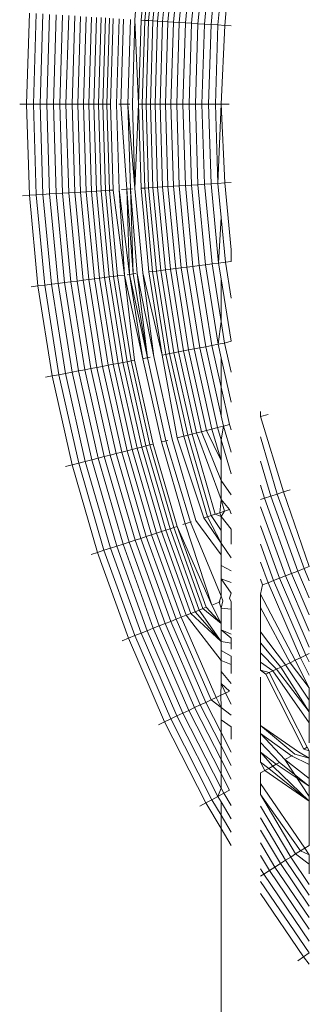
# Model space of a CAD drawing. Units: inches. Extents: x 64 to 1167, y 117 to 939.
# Tile 44 of 56: x 1129.764 to 1129.8616, y 500.6393 to 500.9712. Entities that reach past the tile are written whole.
import ezdxf

# ---------------------------------------------------------------- set-up
doc = ezdxf.new("R2010")
doc.units = ezdxf.units.IN
doc.header["$MEASUREMENT"] = 0
doc.layers.add('A-FLOR-FIXT', color=8, linetype='Continuous', lineweight=18)

msp = doc.modelspace()

# ---------------------------------------------------------------- linework, layer by layer
at = {"layer": 'A-FLOR-FIXT'}
for p, q in [((1129.8047, 500.99961), (1129.80282, 500.97117)), ((1129.80753, 500.99926), (1129.80486, 500.97104)), ((1129.80874, 500.9991), (1129.80608, 500.97096)), ((1129.81007, 500.99893), (1129.80742, 500.97088)), ((1129.81153, 500.99875), (1129.80888, 500.97078)), ((1129.81309, 500.99855), (1129.81046, 500.97069)), ((1129.81477, 500.99834), (1129.81214, 500.97058)), ((1129.81654, 500.99812), (1129.81392, 500.97047)), ((1129.8184, 500.99788), (1129.8158, 500.97035)), ((1129.82034, 500.99764), (1129.81775, 500.97023)), ((1129.82237, 500.99738), (1129.81979, 500.9701)), ((1129.82445, 500.99712), (1129.82189, 500.96997)), ((1129.8266, 500.99685), (1129.82404, 500.96983)), ((1129.82879, 500.99657), (1129.82625, 500.96969)), ((1129.83102, 500.99629), (1129.82849, 500.96955)), ((1129.83328, 500.996), (1129.83077, 500.96941)), ((1129.83519, 500.9918), (1129.83306, 500.96926)), ((1129.76722, 500.97341), (1129.76626, 500.94271)), ((1129.76952, 500.97326), (1129.76856, 500.94271)), ((1129.77179, 500.97312), (1129.77084, 500.94271)), ((1129.77404, 500.97298), (1129.77309, 500.94271)), ((1129.77624, 500.97284), (1129.7753, 500.94271)), ((1129.7784, 500.9727), (1129.77746, 500.94271)), ((1129.7805, 500.97257), (1129.77956, 500.94271)), ((1129.78253, 500.97244), (1129.7816, 500.94271)), ((1129.78449, 500.97232), (1129.78356, 500.94271)), ((1129.78636, 500.9722), (1129.78544, 500.94271)), ((1129.78814, 500.97209), (1129.78722, 500.94271)), ((1129.78983, 500.97198), (1129.78891, 500.94271)), ((1129.7914, 500.97188), (1129.79048, 500.94271)), ((1129.79286, 500.97179), (1129.79195, 500.94271)), ((1129.79421, 500.97171), (1129.7933, 500.94271)), ((1129.79542, 500.97163), (1129.79451, 500.94271)), ((1129.79746, 500.9715), (1129.79656, 500.94271)), ((1129.79894, 500.97141), (1129.79804, 500.94271)), ((1129.80134, 500.97126), (1129.80045, 500.94271)), ((1129.80282, 500.97117), (1129.80193, 500.94271)), ((1129.80282, 500.97117), (1129.80397, 500.94271)), ((1129.80486, 500.97104), (1129.80397, 500.94271)), ((1129.80486, 500.97104), (1129.80608, 500.97096)), ((1129.80608, 500.97096), (1129.80519, 500.94271)), ((1129.80608, 500.97096), (1129.80742, 500.97088)), ((1129.80742, 500.97088), (1129.80654, 500.94271)), ((1129.80742, 500.97088), (1129.80888, 500.97078)), ((1129.80888, 500.97078), (1129.808, 500.94271)), ((1129.80888, 500.97078), (1129.81046, 500.97069)), ((1129.81046, 500.97069), (1129.80958, 500.94271)), ((1129.81046, 500.97069), (1129.81214, 500.97058)), ((1129.81214, 500.97058), (1129.81127, 500.94271)), ((1129.81214, 500.97058), (1129.81392, 500.97047)), ((1129.81392, 500.97047), (1129.81305, 500.94271)), ((1129.81392, 500.97047), (1129.8158, 500.97035)), ((1129.8158, 500.97035), (1129.81493, 500.94271)), ((1129.8158, 500.97035), (1129.81775, 500.97023)), ((1129.81775, 500.97023), (1129.81689, 500.94271)), ((1129.81775, 500.97023), (1129.81979, 500.9701)), ((1129.81979, 500.9701), (1129.81893, 500.94271)), ((1129.81979, 500.9701), (1129.82189, 500.96997)), ((1129.82189, 500.96997), (1129.82103, 500.94271)), ((1129.82189, 500.96997), (1129.82404, 500.96983)), ((1129.82404, 500.96983), (1129.82319, 500.94271)), ((1129.82404, 500.96983), (1129.82625, 500.96969)), ((1129.82625, 500.96969), (1129.8254, 500.94271)), ((1129.82625, 500.96969), (1129.82849, 500.96955)), ((1129.82849, 500.96955), (1129.82765, 500.94271)), ((1129.82849, 500.96955), (1129.83077, 500.96941)), ((1129.83077, 500.96941), (1129.82993, 500.94271)), ((1129.83077, 500.96941), (1129.83306, 500.96926)), ((1129.83306, 500.96926), (1129.83185, 500.94271)), ((1129.83306, 500.96926), (1129.83519, 500.96913)), ((1129.76626, 500.94271), (1129.76395, 500.94271)), ((1129.76626, 500.94271), (1129.76722, 500.91201)), ((1129.76856, 500.94271), (1129.76626, 500.94271)), ((1129.76856, 500.94271), (1129.76952, 500.91215)), ((1129.77084, 500.94271), (1129.76856, 500.94271)), ((1129.77084, 500.94271), (1129.77179, 500.9123)), ((1129.77309, 500.94271), (1129.77084, 500.94271)), ((1129.7753, 500.94271), (1129.77309, 500.94271)), ((1129.77309, 500.94271), (1129.77404, 500.91244)), ((1129.7753, 500.94271), (1129.77624, 500.91258)), ((1129.77746, 500.94271), (1129.7753, 500.94271)), ((1129.77746, 500.94271), (1129.7784, 500.91271)), ((1129.77956, 500.94271), (1129.77746, 500.94271)), ((1129.77956, 500.94271), (1129.7805, 500.91285)), ((1129.7816, 500.94271), (1129.77956, 500.94271)), ((1129.7816, 500.94271), (1129.78253, 500.91297)), ((1129.78356, 500.94271), (1129.7816, 500.94271)), ((1129.78544, 500.94271), (1129.78356, 500.94271)), ((1129.78356, 500.94271), (1129.78449, 500.9131)), ((1129.78722, 500.94271), (1129.78544, 500.94271)), ((1129.78544, 500.94271), (1129.78636, 500.91321)), ((1129.78722, 500.94271), (1129.78814, 500.91333)), ((1129.78891, 500.94271), (1129.78722, 500.94271)), ((1129.78891, 500.94271), (1129.78983, 500.91343)), ((1129.79048, 500.94271), (1129.78891, 500.94271)), ((1129.79048, 500.94271), (1129.7914, 500.91353)), ((1129.79195, 500.94271), (1129.79048, 500.94271)), ((1129.79195, 500.94271), (1129.79286, 500.91362)), ((1129.7933, 500.94271), (1129.79195, 500.94271)), ((1129.7933, 500.94271), (1129.79421, 500.91371)), ((1129.79451, 500.94271), (1129.7933, 500.94271)), ((1129.79451, 500.94271), (1129.79542, 500.91378)), ((1129.79656, 500.94271), (1129.79746, 500.91391)), ((1129.79737, 500.94271), (1129.80112, 500.94271)), ((1129.79804, 500.94271), (1129.80007, 500.91408)), ((1129.80045, 500.94271), (1129.80282, 500.91425)), ((1129.80045, 500.94271), (1129.80134, 500.91416)), ((1129.80193, 500.94271), (1129.80282, 500.91425)), ((1129.80397, 500.94271), (1129.80282, 500.91425)), ((1129.80519, 500.94271), (1129.80397, 500.94271)), ((1129.80397, 500.94271), (1129.80486, 500.91438)), ((1129.80519, 500.94271), (1129.80608, 500.91445)), ((1129.80654, 500.94271), (1129.80519, 500.94271)), ((1129.808, 500.94271), (1129.80654, 500.94271)), ((1129.80654, 500.94271), (1129.80742, 500.91454)), ((1129.80958, 500.94271), (1129.808, 500.94271)), ((1129.808, 500.94271), (1129.80888, 500.91463)), ((1129.81127, 500.94271), (1129.80958, 500.94271)), ((1129.80958, 500.94271), (1129.81046, 500.91473)), ((1129.81305, 500.94271), (1129.81127, 500.94271)), ((1129.81127, 500.94271), (1129.81214, 500.91484)), ((1129.81305, 500.94271), (1129.81392, 500.91495)), ((1129.81493, 500.94271), (1129.81305, 500.94271)), ((1129.81493, 500.94271), (1129.8158, 500.91507)), ((1129.81689, 500.94271), (1129.81493, 500.94271)), ((1129.81893, 500.94271), (1129.81689, 500.94271)), ((1129.81689, 500.94271), (1129.81775, 500.91519)), ((1129.82103, 500.94271), (1129.81893, 500.94271)), ((1129.81893, 500.94271), (1129.81979, 500.91532)), ((1129.82319, 500.94271), (1129.82103, 500.94271)), ((1129.82103, 500.94271), (1129.82189, 500.91545)), ((1129.8254, 500.94271), (1129.82319, 500.94271)), ((1129.82319, 500.94271), (1129.82404, 500.91558)), ((1129.82765, 500.94271), (1129.8254, 500.94271)), ((1129.8254, 500.94271), (1129.82625, 500.91572)), ((1129.82993, 500.94271), (1129.82765, 500.94271)), ((1129.82765, 500.94271), (1129.82849, 500.91586)), ((1129.83185, 500.94271), (1129.82993, 500.94271)), ((1129.82993, 500.94271), (1129.83077, 500.91601)), ((1129.83077, 500.91601), (1129.83185, 500.94271)), ((1129.83454, 500.94271), (1129.83185, 500.94271)), ((1129.83185, 500.94271), (1129.83306, 500.91615)), ((1129.78449, 500.9131), (1129.78253, 500.91297)), ((1129.78636, 500.91321), (1129.78449, 500.9131)), ((1129.78449, 500.9131), (1129.78728, 500.8836)), ((1129.78814, 500.91333), (1129.78636, 500.91321)), ((1129.78636, 500.91321), (1129.78914, 500.88384)), ((1129.78983, 500.91343), (1129.78814, 500.91333)), ((1129.78814, 500.91333), (1129.79091, 500.88406)), ((1129.7914, 500.91353), (1129.78983, 500.91343)), ((1129.78983, 500.91343), (1129.79258, 500.88427)), ((1129.79286, 500.91362), (1129.7914, 500.91353)), ((1129.7914, 500.91353), (1129.79415, 500.88447)), ((1129.79421, 500.91371), (1129.79286, 500.91362)), ((1129.79286, 500.91362), (1129.7956, 500.88465)), ((1129.79542, 500.91378), (1129.79421, 500.91371)), ((1129.79421, 500.91371), (1129.79694, 500.88482)), ((1129.79542, 500.91378), (1129.79923, 500.88511)), ((1129.79746, 500.91391), (1129.79923, 500.88511)), ((1129.79746, 500.91391), (1129.80098, 500.88533)), ((1129.79827, 500.91396), (1129.80201, 500.9142)), ((1129.80007, 500.91408), (1129.80217, 500.88548)), ((1129.80007, 500.91408), (1129.80098, 500.88533)), ((1129.80134, 500.91416), (1129.80351, 500.88565)), ((1129.80134, 500.91416), (1129.80217, 500.88548)), ((1129.80282, 500.91425), (1129.8055, 500.8859)), ((1129.80608, 500.91445), (1129.80486, 500.91438)), ((1129.80486, 500.91438), (1129.80753, 500.88616)), ((1129.80742, 500.91454), (1129.80608, 500.91445)), ((1129.80608, 500.91445), (1129.80874, 500.88631)), ((1129.80888, 500.91463), (1129.80742, 500.91454)), ((1129.80742, 500.91454), (1129.81007, 500.88648)), ((1129.81046, 500.91473), (1129.80888, 500.91463)), ((1129.80888, 500.91463), (1129.81153, 500.88666)), ((1129.81214, 500.91484), (1129.81046, 500.91473)), ((1129.81046, 500.91473), (1129.81309, 500.88686)), ((1129.81392, 500.91495), (1129.81214, 500.91484)), ((1129.81214, 500.91484), (1129.81477, 500.88707)), ((1129.8158, 500.91507), (1129.81392, 500.91495)), ((1129.81392, 500.91495), (1129.81654, 500.8873)), ((1129.81775, 500.91519), (1129.8158, 500.91507)), ((1129.8158, 500.91507), (1129.8184, 500.88753)), ((1129.81979, 500.91532), (1129.81775, 500.91519)), ((1129.81775, 500.91519), (1129.82034, 500.88778)), ((1129.82189, 500.91545), (1129.81979, 500.91532)), ((1129.81979, 500.91532), (1129.82237, 500.88803)), ((1129.82404, 500.91558), (1129.82189, 500.91545)), ((1129.82189, 500.91545), (1129.82445, 500.8883)), ((1129.82625, 500.91572), (1129.82404, 500.91558)), ((1129.82404, 500.91558), (1129.8266, 500.88857)), ((1129.82849, 500.91586), (1129.82625, 500.91572)), ((1129.82625, 500.91572), (1129.82879, 500.88885)), ((1129.83077, 500.91601), (1129.82849, 500.91586)), ((1129.82849, 500.91586), (1129.83102, 500.88913)), ((1129.83306, 500.91615), (1129.83077, 500.91601)), ((1129.83077, 500.91601), (1129.83185, 500.90452)), ((1129.83519, 500.91629), (1129.83306, 500.91615)), ((1129.83306, 500.91615), (1129.83519, 500.89362)), ((1129.76722, 500.91201), (1129.76492, 500.91186)), ((1129.76952, 500.91215), (1129.76722, 500.91201)), ((1129.76722, 500.91201), (1129.77011, 500.88143)), ((1129.77179, 500.9123), (1129.76952, 500.91215)), ((1129.76952, 500.91215), (1129.77239, 500.88172)), ((1129.77404, 500.91244), (1129.77179, 500.9123)), ((1129.77179, 500.9123), (1129.77465, 500.88201)), ((1129.77624, 500.91258), (1129.77404, 500.91244)), ((1129.77404, 500.91244), (1129.77689, 500.88229)), ((1129.7784, 500.91271), (1129.77624, 500.91258)), ((1129.77624, 500.91258), (1129.77908, 500.88257)), ((1129.7805, 500.91285), (1129.7784, 500.91271)), ((1129.7784, 500.91271), (1129.78122, 500.88284)), ((1129.78253, 500.91297), (1129.7805, 500.91285)), ((1129.7805, 500.91285), (1129.78331, 500.8831)), ((1129.78253, 500.91297), (1129.78533, 500.88336)), ((1129.83102, 500.88913), (1129.83185, 500.90452)), ((1129.83185, 500.90452), (1129.83328, 500.88941)), ((1129.83519, 500.89362), (1129.83519, 500.88965)), ((1129.81153, 500.88666), (1129.81007, 500.88648)), ((1129.81309, 500.88686), (1129.81153, 500.88666)), ((1129.81153, 500.88666), (1129.81592, 500.85892)), ((1129.81477, 500.88707), (1129.81309, 500.88686)), ((1129.81309, 500.88686), (1129.81747, 500.85922)), ((1129.81654, 500.8873), (1129.81477, 500.88707)), ((1129.81477, 500.88707), (1129.81913, 500.85953)), ((1129.8184, 500.88753), (1129.81654, 500.8873)), ((1129.81654, 500.8873), (1129.82088, 500.85987)), ((1129.82034, 500.88778), (1129.8184, 500.88753)), ((1129.8184, 500.88753), (1129.82273, 500.86022)), ((1129.82237, 500.88803), (1129.82034, 500.88778)), ((1129.82034, 500.88778), (1129.82465, 500.86059)), ((1129.82445, 500.8883), (1129.82237, 500.88803)), ((1129.82237, 500.88803), (1129.82665, 500.86097)), ((1129.8266, 500.88857), (1129.82445, 500.8883)), ((1129.82445, 500.8883), (1129.82872, 500.86136)), ((1129.82879, 500.88885), (1129.8266, 500.88857)), ((1129.8266, 500.88857), (1129.83084, 500.86177)), ((1129.83102, 500.88913), (1129.82879, 500.88885)), ((1129.82879, 500.88885), (1129.83185, 500.8695)), ((1129.83328, 500.88941), (1129.83102, 500.88913)), ((1129.83102, 500.88913), (1129.83185, 500.88387)), ((1129.83519, 500.88965), (1129.83328, 500.88941)), ((1129.83328, 500.88941), (1129.83519, 500.87735)), ((1129.78533, 500.88336), (1129.78331, 500.8831)), ((1129.78728, 500.8836), (1129.78533, 500.88336)), ((1129.78533, 500.88336), (1129.78998, 500.85397)), ((1129.78914, 500.88384), (1129.78728, 500.8836)), ((1129.78728, 500.8836), (1129.79191, 500.85434)), ((1129.79091, 500.88406), (1129.78914, 500.88384)), ((1129.78914, 500.88384), (1129.79376, 500.85469)), ((1129.79258, 500.88427), (1129.79091, 500.88406)), ((1129.79091, 500.88406), (1129.79551, 500.85503)), ((1129.79415, 500.88447), (1129.79258, 500.88427)), ((1129.79258, 500.88427), (1129.79716, 500.85534)), ((1129.7956, 500.88465), (1129.79415, 500.88447)), ((1129.79415, 500.88447), (1129.79872, 500.85564)), ((1129.79694, 500.88482), (1129.7956, 500.88465)), ((1129.7956, 500.88465), (1129.80015, 500.85591)), ((1129.79923, 500.88511), (1129.79694, 500.88482)), ((1129.79694, 500.88482), (1129.80148, 500.85616)), ((1129.79923, 500.88511), (1129.80267, 500.85639)), ((1129.79923, 500.88511), (1129.80548, 500.85693)), ((1129.80017, 500.88523), (1129.80314, 500.88561)), ((1129.80098, 500.88533), (1129.80548, 500.85693)), ((1129.80098, 500.88533), (1129.80702, 500.85722)), ((1129.80217, 500.88548), (1129.80702, 500.85722)), ((1129.80351, 500.88565), (1129.80916, 500.85763)), ((1129.80351, 500.88565), (1129.80702, 500.85722)), ((1129.8055, 500.8859), (1129.80916, 500.85763)), ((1129.8055, 500.8859), (1129.81196, 500.85816)), ((1129.80874, 500.88631), (1129.80753, 500.88616)), ((1129.80753, 500.88616), (1129.81196, 500.85816)), ((1129.81007, 500.88648), (1129.80874, 500.88631)), ((1129.80874, 500.88631), (1129.81316, 500.85839)), ((1129.81007, 500.88648), (1129.81448, 500.85865)), ((1129.83185, 500.88387), (1129.83519, 500.86279)), ((1129.83185, 500.8695), (1129.83185, 500.88387)), ((1129.77011, 500.88143), (1129.76782, 500.88114)), ((1129.77239, 500.88172), (1129.77011, 500.88143)), ((1129.77011, 500.88143), (1129.77492, 500.8511)), ((1129.77465, 500.88201), (1129.77239, 500.88172)), ((1129.77239, 500.88172), (1129.77718, 500.85153)), ((1129.77689, 500.88229), (1129.77465, 500.88201)), ((1129.77465, 500.88201), (1129.77941, 500.85196)), ((1129.77908, 500.88257), (1129.77689, 500.88229)), ((1129.77689, 500.88229), (1129.78162, 500.85238)), ((1129.78122, 500.88284), (1129.77908, 500.88257)), ((1129.77908, 500.88257), (1129.78379, 500.85279)), ((1129.78331, 500.8831), (1129.78122, 500.88284)), ((1129.78122, 500.88284), (1129.78592, 500.8532)), ((1129.78331, 500.8831), (1129.78798, 500.85359)), ((1129.83084, 500.86177), (1129.83185, 500.8695)), ((1129.83185, 500.8695), (1129.83301, 500.86218)), ((1129.82273, 500.86022), (1129.82088, 500.85987)), ((1129.82465, 500.86059), (1129.82273, 500.86022)), ((1129.82273, 500.86022), (1129.82876, 500.83323)), ((1129.82665, 500.86097), (1129.82465, 500.86059)), ((1129.82465, 500.86059), (1129.83066, 500.83372)), ((1129.82872, 500.86136), (1129.82665, 500.86097)), ((1129.82665, 500.86097), (1129.83185, 500.8377)), ((1129.83084, 500.86177), (1129.82872, 500.86136)), ((1129.82872, 500.86136), (1129.83185, 500.84734)), ((1129.83301, 500.86218), (1129.83084, 500.86177)), ((1129.83084, 500.86177), (1129.83185, 500.85724)), ((1129.83519, 500.86279), (1129.83301, 500.86218)), ((1129.83301, 500.86218), (1129.83519, 500.85243)), ((1129.80548, 500.85693), (1129.81175, 500.82886)), ((1129.80571, 500.85697), (1129.80798, 500.85741)), ((1129.80702, 500.85722), (1129.81327, 500.82925)), ((1129.80916, 500.85763), (1129.81538, 500.82979)), ((1129.81316, 500.85839), (1129.81196, 500.85816)), ((1129.81196, 500.85816), (1129.81709, 500.83023)), ((1129.81448, 500.85865), (1129.81316, 500.85839)), ((1129.81316, 500.85839), (1129.81933, 500.83081)), ((1129.81592, 500.85892), (1129.81448, 500.85865)), ((1129.81448, 500.85865), (1129.82063, 500.83114)), ((1129.81747, 500.85922), (1129.81592, 500.85892)), ((1129.81592, 500.85892), (1129.82205, 500.83151)), ((1129.81913, 500.85953), (1129.81747, 500.85922)), ((1129.81747, 500.85922), (1129.82358, 500.8319)), ((1129.82088, 500.85987), (1129.81913, 500.85953)), ((1129.81913, 500.85953), (1129.82521, 500.83232)), ((1129.82088, 500.85987), (1129.82694, 500.83276)), ((1129.83185, 500.85724), (1129.83519, 500.84231)), ((1129.83185, 500.84734), (1129.83185, 500.85724)), ((1129.78798, 500.85359), (1129.78592, 500.8532)), ((1129.78998, 500.85397), (1129.78798, 500.85359)), ((1129.78798, 500.85359), (1129.7945, 500.82443)), ((1129.79191, 500.85434), (1129.78998, 500.85397)), ((1129.78998, 500.85397), (1129.79647, 500.82494)), ((1129.79376, 500.85469), (1129.79191, 500.85434)), ((1129.79191, 500.85434), (1129.79837, 500.82543)), ((1129.79551, 500.85503), (1129.79376, 500.85469)), ((1129.79376, 500.85469), (1129.80019, 500.82589)), ((1129.79716, 500.85534), (1129.79551, 500.85503)), ((1129.79551, 500.85503), (1129.80192, 500.82634)), ((1129.79872, 500.85564), (1129.79716, 500.85534)), ((1129.79716, 500.85534), (1129.80355, 500.82676)), ((1129.80015, 500.85591), (1129.79872, 500.85564)), ((1129.79872, 500.85564), (1129.80508, 500.82715)), ((1129.80148, 500.85616), (1129.80015, 500.85591)), ((1129.80015, 500.85591), (1129.8065, 500.82751)), ((1129.80267, 500.85639), (1129.80148, 500.85616)), ((1129.80148, 500.85616), (1129.80781, 500.82785)), ((1129.80267, 500.85639), (1129.80899, 500.82815)), ((1129.77492, 500.8511), (1129.77265, 500.85067)), ((1129.77718, 500.85153), (1129.77492, 500.8511)), ((1129.77492, 500.8511), (1129.78162, 500.82113)), ((1129.77941, 500.85196), (1129.77718, 500.85153)), ((1129.77718, 500.85153), (1129.78384, 500.8217)), ((1129.78162, 500.85238), (1129.77941, 500.85196)), ((1129.77941, 500.85196), (1129.78605, 500.82226)), ((1129.78379, 500.85279), (1129.78162, 500.85238)), ((1129.78162, 500.85238), (1129.78823, 500.82282)), ((1129.78592, 500.8532), (1129.78379, 500.85279)), ((1129.78379, 500.85279), (1129.79037, 500.82337)), ((1129.78592, 500.8532), (1129.79246, 500.82391)), ((1129.83185, 500.84734), (1129.83467, 500.83475)), ((1129.83185, 500.8377), (1129.83185, 500.84734)), ((1129.83185, 500.8377), (1129.83263, 500.83422)), ((1129.84515, 500.83915), (1129.84515, 500.83744)), ((1129.84775, 500.8381), (1129.84515, 500.83744)), ((1129.84515, 500.83744), (1129.85293, 500.81202)), ((1129.83066, 500.83372), (1129.82876, 500.83323)), ((1129.83263, 500.83422), (1129.83066, 500.83372)), ((1129.83066, 500.83372), (1129.83185, 500.8296)), ((1129.83185, 500.8296), (1129.83263, 500.83422)), ((1129.83467, 500.83475), (1129.83263, 500.83422)), ((1129.83263, 500.83422), (1129.83519, 500.82541)), ((1129.83467, 500.83475), (1129.83519, 500.83294)), ((1129.81933, 500.83081), (1129.81709, 500.83023)), ((1129.81709, 500.83023), (1129.82605, 500.80329)), ((1129.82063, 500.83114), (1129.81933, 500.83081)), ((1129.81933, 500.83081), (1129.82721, 500.80366)), ((1129.82205, 500.83151), (1129.82063, 500.83114)), ((1129.82063, 500.83114), (1129.82849, 500.80408)), ((1129.82358, 500.8319), (1129.82205, 500.83151)), ((1129.82205, 500.83151), (1129.82989, 500.80453)), ((1129.82521, 500.83232), (1129.82358, 500.8319)), ((1129.82358, 500.8319), (1129.83185, 500.80945)), ((1129.82694, 500.83276), (1129.82521, 500.83232)), ((1129.82521, 500.83232), (1129.83185, 500.81585)), ((1129.82876, 500.83323), (1129.82694, 500.83276)), ((1129.82694, 500.83276), (1129.83185, 500.82257)), ((1129.82876, 500.83323), (1129.83185, 500.82257)), ((1129.84515, 500.83054), (1129.85074, 500.81131)), ((1129.80355, 500.82676), (1129.80508, 500.82715)), ((1129.80508, 500.82715), (1129.8065, 500.82751)), ((1129.80508, 500.82715), (1129.81323, 500.79912)), ((1129.8065, 500.82751), (1129.80781, 500.82785)), ((1129.8065, 500.82751), (1129.81462, 500.79957)), ((1129.80781, 500.82785), (1129.80899, 500.82815)), ((1129.80781, 500.82785), (1129.8159, 500.79999)), ((1129.80899, 500.82815), (1129.81706, 500.80036)), ((1129.81175, 500.82886), (1129.81978, 500.80125)), ((1129.8119, 500.8289), (1129.81386, 500.8294)), ((1129.81327, 500.82925), (1129.82148, 500.8018)), ((1129.81538, 500.82979), (1129.82334, 500.8024)), ((1129.83185, 500.8296), (1129.83519, 500.81811)), ((1129.83185, 500.82257), (1129.83185, 500.8296)), ((1129.79037, 500.82337), (1129.79246, 500.82391)), ((1129.79246, 500.82391), (1129.7945, 500.82443)), ((1129.79246, 500.82391), (1129.80084, 500.79509)), ((1129.7945, 500.82443), (1129.79647, 500.82494)), ((1129.7945, 500.82443), (1129.80284, 500.79574)), ((1129.79647, 500.82494), (1129.79837, 500.82543)), ((1129.79647, 500.82494), (1129.80477, 500.79637)), ((1129.79837, 500.82543), (1129.80019, 500.82589)), ((1129.79837, 500.82543), (1129.80664, 500.79698)), ((1129.80019, 500.82589), (1129.80192, 500.82634)), ((1129.80019, 500.82589), (1129.80842, 500.79756)), ((1129.80192, 500.82634), (1129.80355, 500.82676)), ((1129.80192, 500.82634), (1129.81012, 500.79811)), ((1129.80355, 500.82676), (1129.81173, 500.79863)), ((1129.77938, 500.82055), (1129.78162, 500.82113)), ((1129.78162, 500.82113), (1129.78384, 500.8217)), ((1129.78162, 500.82113), (1129.79019, 500.79163)), ((1129.78384, 500.8217), (1129.78605, 500.82226)), ((1129.78384, 500.8217), (1129.79237, 500.79234)), ((1129.78605, 500.82226), (1129.78823, 500.82282)), ((1129.78605, 500.82226), (1129.79454, 500.79305)), ((1129.78823, 500.82282), (1129.79037, 500.82337)), ((1129.78823, 500.82282), (1129.79668, 500.79374)), ((1129.79037, 500.82337), (1129.79878, 500.79442)), ((1129.83185, 500.82257), (1129.83185, 500.81585)), ((1129.84515, 500.82238), (1129.84857, 500.8106)), ((1129.83185, 500.81585), (1129.83519, 500.81108)), ((1129.83185, 500.81585), (1129.83185, 500.80945)), ((1129.84515, 500.81432), (1129.84643, 500.80991)), ((1129.84857, 500.8106), (1129.84643, 500.80991)), ((1129.85074, 500.81131), (1129.84857, 500.8106)), ((1129.84857, 500.8106), (1129.85767, 500.78533)), ((1129.85293, 500.81202), (1129.85074, 500.81131)), ((1129.85074, 500.81131), (1129.85979, 500.78617)), ((1129.85512, 500.81273), (1129.85293, 500.81202)), ((1129.85293, 500.81202), (1129.86158, 500.78688)), ((1129.83185, 500.80945), (1129.83139, 500.80502)), ((1129.83185, 500.80945), (1129.83469, 500.80609)), ((1129.83185, 500.80945), (1129.83299, 500.80554)), ((1129.84643, 500.80991), (1129.84515, 500.80949)), ((1129.84515, 500.80695), (1129.85352, 500.78369)), ((1129.84643, 500.80991), (1129.85558, 500.78451)), ((1129.82721, 500.80366), (1129.82605, 500.80329)), ((1129.82849, 500.80408), (1129.82721, 500.80366)), ((1129.82721, 500.80366), (1129.83185, 500.79474)), ((1129.82989, 500.80453), (1129.82849, 500.80408)), ((1129.82849, 500.80408), (1129.83185, 500.79907)), ((1129.83139, 500.80502), (1129.82989, 500.80453)), ((1129.82989, 500.80453), (1129.83185, 500.80372)), ((1129.83299, 500.80554), (1129.83139, 500.80502)), ((1129.83139, 500.80502), (1129.83185, 500.80372)), ((1129.83299, 500.80554), (1129.83185, 500.80372)), ((1129.83185, 500.80372), (1129.83519, 500.79943)), ((1129.83185, 500.80372), (1129.83185, 500.79907)), ((1129.83469, 500.80609), (1129.83299, 500.80554)), ((1129.83469, 500.80609), (1129.83519, 500.80469)), ((1129.8159, 500.79999), (1129.81706, 500.80036)), ((1129.81706, 500.80036), (1129.82686, 500.77314)), ((1129.81706, 500.80036), (1129.82876, 500.77389)), ((1129.819, 500.80099), (1129.82184, 500.80192)), ((1129.81978, 500.80125), (1129.82876, 500.77389)), ((1129.82148, 500.8018), (1129.83185, 500.77689)), ((1129.82334, 500.8024), (1129.83185, 500.79077)), ((1129.82605, 500.80329), (1129.83185, 500.79474)), ((1129.84515, 500.80057), (1129.85151, 500.7829)), ((1129.80477, 500.79637), (1129.80664, 500.79698)), ((1129.80664, 500.79698), (1129.80842, 500.79756)), ((1129.80664, 500.79698), (1129.81667, 500.7691)), ((1129.80842, 500.79756), (1129.81012, 500.79811)), ((1129.80842, 500.79756), (1129.81842, 500.76979)), ((1129.81012, 500.79811), (1129.81173, 500.79863)), ((1129.81012, 500.79811), (1129.82008, 500.77045)), ((1129.81173, 500.79863), (1129.81323, 500.79912)), ((1129.81173, 500.79863), (1129.82165, 500.77107)), ((1129.81323, 500.79912), (1129.81462, 500.79957)), ((1129.81323, 500.79912), (1129.82312, 500.77165)), ((1129.81462, 500.79957), (1129.8159, 500.79999)), ((1129.81462, 500.79957), (1129.82448, 500.77219)), ((1129.8159, 500.79999), (1129.82573, 500.77269)), ((1129.83185, 500.79907), (1129.83185, 500.79474)), ((1129.83519, 500.79943), (1129.83519, 500.79445)), ((1129.79454, 500.79305), (1129.79668, 500.79374)), ((1129.79668, 500.79374), (1129.79878, 500.79442)), ((1129.79668, 500.79374), (1129.80694, 500.76525)), ((1129.79878, 500.79442), (1129.80084, 500.79509)), ((1129.79878, 500.79442), (1129.80899, 500.76606)), ((1129.80084, 500.79509), (1129.80284, 500.79574)), ((1129.80084, 500.79509), (1129.811, 500.76686)), ((1129.80284, 500.79574), (1129.80477, 500.79637)), ((1129.80284, 500.79574), (1129.81296, 500.76763)), ((1129.80477, 500.79637), (1129.81485, 500.76838)), ((1129.83185, 500.79474), (1129.83519, 500.78979)), ((1129.83185, 500.79474), (1129.83185, 500.79077)), ((1129.84515, 500.79436), (1129.84956, 500.78212)), ((1129.78799, 500.79092), (1129.79019, 500.79163)), ((1129.79019, 500.79163), (1129.79237, 500.79234)), ((1129.79019, 500.79163), (1129.80059, 500.76273)), ((1129.79237, 500.79234), (1129.79454, 500.79305)), ((1129.79237, 500.79234), (1129.80273, 500.76358)), ((1129.79454, 500.79305), (1129.80485, 500.76442)), ((1129.83185, 500.79077), (1129.83185, 500.78717)), ((1129.83185, 500.78717), (1129.83519, 500.78547)), ((1129.83185, 500.78717), (1129.83185, 500.78268)), ((1129.84515, 500.78835), (1129.84767, 500.78137)), ((1129.85352, 500.78369), (1129.85151, 500.7829)), ((1129.85558, 500.78451), (1129.85352, 500.78369)), ((1129.85352, 500.78369), (1129.86158, 500.76508)), ((1129.85767, 500.78533), (1129.85558, 500.78451)), ((1129.85558, 500.78451), (1129.86158, 500.77064)), ((1129.85979, 500.78617), (1129.85767, 500.78533)), ((1129.85767, 500.78533), (1129.86158, 500.7763)), ((1129.86158, 500.78688), (1129.85979, 500.78617)), ((1129.85979, 500.78617), (1129.86158, 500.78204)), ((1129.83185, 500.78268), (1129.83519, 500.7779)), ((1129.83185, 500.78268), (1129.83185, 500.77689)), ((1129.83185, 500.78268), (1129.83519, 500.7815)), ((1129.84515, 500.78257), (1129.84584, 500.78065)), ((1129.84584, 500.78065), (1129.84515, 500.77752)), ((1129.84767, 500.78137), (1129.84584, 500.78065)), ((1129.84956, 500.78212), (1129.84767, 500.78137)), ((1129.84767, 500.78137), (1129.8586, 500.7561)), ((1129.85151, 500.7829), (1129.84956, 500.78212)), ((1129.84956, 500.78212), (1129.86044, 500.75697)), ((1129.85151, 500.7829), (1129.86158, 500.75964)), ((1129.83519, 500.7779), (1129.83464, 500.77622)), ((1129.84515, 500.77752), (1129.84515, 500.77303)), ((1129.84515, 500.77752), (1129.85683, 500.75527)), ((1129.82876, 500.77389), (1129.83154, 500.77499)), ((1129.82876, 500.77389), (1129.83185, 500.76772)), ((1129.83185, 500.77689), (1129.83119, 500.77485)), ((1129.83119, 500.77485), (1129.83185, 500.77284)), ((1129.83185, 500.77689), (1129.83238, 500.77532)), ((1129.83238, 500.77532), (1129.83185, 500.77284)), ((1129.83464, 500.77622), (1129.83519, 500.77495)), ((1129.83519, 500.77495), (1129.83519, 500.77255)), ((1129.82008, 500.77045), (1129.81842, 500.76979)), ((1129.82165, 500.77107), (1129.82008, 500.77045)), ((1129.82008, 500.77045), (1129.83185, 500.75515)), ((1129.82312, 500.77165), (1129.82165, 500.77107)), ((1129.82165, 500.77107), (1129.83185, 500.7616)), ((1129.82448, 500.77219), (1129.82312, 500.77165)), ((1129.82312, 500.77165), (1129.83185, 500.7616)), ((1129.82573, 500.77269), (1129.82448, 500.77219)), ((1129.82448, 500.77219), (1129.83185, 500.7616)), ((1129.82686, 500.77314), (1129.82573, 500.77269)), ((1129.82573, 500.77269), (1129.83185, 500.76772)), ((1129.82686, 500.77314), (1129.83185, 500.76772)), ((1129.83185, 500.77284), (1129.83185, 500.76772)), ((1129.83185, 500.77284), (1129.83519, 500.77255)), ((1129.83519, 500.77255), (1129.83519, 500.7705)), ((1129.83519, 500.7705), (1129.83519, 500.76881)), ((1129.83519, 500.7656), (1129.83519, 500.7705)), ((1129.84515, 500.77303), (1129.85513, 500.75447)), ((1129.84515, 500.76481), (1129.84515, 500.77303)), ((1129.81296, 500.76763), (1129.811, 500.76686)), ((1129.81485, 500.76838), (1129.81296, 500.76763)), ((1129.81296, 500.76763), (1129.82482, 500.74021)), ((1129.81667, 500.7691), (1129.81485, 500.76838)), ((1129.81485, 500.76838), (1129.82667, 500.74108)), ((1129.81842, 500.76979), (1129.81667, 500.7691)), ((1129.81667, 500.7691), (1129.82844, 500.74191)), ((1129.81842, 500.76979), (1129.83014, 500.74271)), ((1129.83185, 500.76772), (1129.83185, 500.76559)), ((1129.80485, 500.76442), (1129.80273, 500.76358)), ((1129.80694, 500.76525), (1129.80485, 500.76442)), ((1129.80485, 500.76442), (1129.81693, 500.7365)), ((1129.80899, 500.76606), (1129.80694, 500.76525)), ((1129.80694, 500.76525), (1129.81896, 500.73745)), ((1129.811, 500.76686), (1129.80899, 500.76606)), ((1129.80899, 500.76606), (1129.82096, 500.73839)), ((1129.811, 500.76686), (1129.82292, 500.73932)), ((1129.83185, 500.76559), (1129.83185, 500.7616)), ((1129.83185, 500.76559), (1129.83519, 500.76276)), ((1129.83185, 500.76559), (1129.83519, 500.76408)), ((1129.84515, 500.76481), (1129.84515, 500.76112)), ((1129.84515, 500.76481), (1129.85351, 500.75371)), ((1129.80059, 500.76273), (1129.79844, 500.76188)), ((1129.80273, 500.76358), (1129.80059, 500.76273)), ((1129.80059, 500.76273), (1129.81279, 500.73455)), ((1129.80273, 500.76358), (1129.81487, 500.73553)), ((1129.83185, 500.7616), (1129.83185, 500.75853)), ((1129.83185, 500.7616), (1129.83519, 500.76107)), ((1129.83519, 500.76276), (1129.83519, 500.76107)), ((1129.83519, 500.76107), (1129.83519, 500.75903)), ((1129.84515, 500.76112), (1129.84515, 500.75774)), ((1129.84515, 500.76112), (1129.85199, 500.75299)), ((1129.83185, 500.75853), (1129.83185, 500.75515)), ((1129.83185, 500.75853), (1129.83519, 500.75663)), ((1129.84515, 500.75774), (1129.84515, 500.75467)), ((1129.84515, 500.75774), (1129.85056, 500.75232)), ((1129.86158, 500.75751), (1129.86044, 500.75697)), ((1129.83185, 500.75515), (1129.83185, 500.75146)), ((1129.83185, 500.75515), (1129.83519, 500.75389)), ((1129.83519, 500.75663), (1129.83519, 500.75389)), ((1129.83519, 500.75389), (1129.83519, 500.75082)), ((1129.84515, 500.75467), (1129.84515, 500.75193)), ((1129.84515, 500.75467), (1129.84923, 500.7517)), ((1129.85513, 500.75447), (1129.85351, 500.75371)), ((1129.85683, 500.75527), (1129.85513, 500.75447)), ((1129.85513, 500.75447), (1129.86158, 500.74594)), ((1129.8586, 500.7561), (1129.85683, 500.75527)), ((1129.85683, 500.75527), (1129.86158, 500.74594)), ((1129.86044, 500.75697), (1129.8586, 500.7561)), ((1129.8586, 500.7561), (1129.86158, 500.75026)), ((1129.86044, 500.75697), (1129.86158, 500.75474)), ((1129.83185, 500.75146), (1129.83519, 500.74743)), ((1129.83185, 500.75146), (1129.83185, 500.74749)), ((1129.84515, 500.75193), (1129.84691, 500.7506)), ((1129.84515, 500.75193), (1129.84801, 500.75112)), ((1129.84691, 500.7506), (1129.84801, 500.75112)), ((1129.84691, 500.7506), (1129.85978, 500.72535)), ((1129.84923, 500.7517), (1129.84801, 500.75112)), ((1129.84801, 500.75112), (1129.86085, 500.72594)), ((1129.85056, 500.75232), (1129.84923, 500.7517)), ((1129.84923, 500.7517), (1129.86158, 500.73417)), ((1129.85199, 500.75299), (1129.85056, 500.75232)), ((1129.85056, 500.75232), (1129.86158, 500.73788)), ((1129.85351, 500.75371), (1129.85199, 500.75299)), ((1129.85199, 500.75299), (1129.86158, 500.73788)), ((1129.85351, 500.75371), (1129.86158, 500.74181)), ((1129.83185, 500.74749), (1129.83175, 500.74347)), ((1129.83185, 500.74749), (1129.83328, 500.74419)), ((1129.83185, 500.74749), (1129.83471, 500.74486)), ((1129.84515, 500.74956), (1129.84515, 500.74348)), ((1129.84515, 500.74348), (1129.84515, 500.74777)), ((1129.83328, 500.74419), (1129.83175, 500.74347)), ((1129.83471, 500.74486), (1129.83328, 500.74419)), ((1129.83328, 500.74419), (1129.83519, 500.74044)), ((1129.86158, 500.74594), (1129.86158, 500.74181)), ((1129.82667, 500.74108), (1129.82482, 500.74021)), ((1129.82844, 500.74191), (1129.82667, 500.74108)), ((1129.82667, 500.74108), (1129.83185, 500.7309)), ((1129.83014, 500.74271), (1129.82844, 500.74191)), ((1129.82844, 500.74191), (1129.83185, 500.73935)), ((1129.83175, 500.74347), (1129.83014, 500.74271)), ((1129.83014, 500.74271), (1129.83185, 500.73935)), ((1129.83175, 500.74347), (1129.83185, 500.73935)), ((1129.84515, 500.74348), (1129.84515, 500.73952)), ((1129.84515, 500.74215), (1129.84515, 500.73952)), ((1129.86158, 500.74181), (1129.86158, 500.73788)), ((1129.81896, 500.73745), (1129.81693, 500.7365)), ((1129.82096, 500.73839), (1129.81896, 500.73745)), ((1129.81896, 500.73745), (1129.83185, 500.71216)), ((1129.82292, 500.73932), (1129.82096, 500.73839)), ((1129.82096, 500.73839), (1129.83185, 500.71702)), ((1129.82482, 500.74021), (1129.82292, 500.73932)), ((1129.82292, 500.73932), (1129.83185, 500.72178)), ((1129.82482, 500.74021), (1129.83185, 500.72641)), ((1129.83185, 500.73935), (1129.83519, 500.73673)), ((1129.83185, 500.73935), (1129.83185, 500.73521)), ((1129.84515, 500.73952), (1129.84515, 500.73324)), ((1129.86158, 500.73788), (1129.86158, 500.73417)), ((1129.81279, 500.73455), (1129.8107, 500.73356)), ((1129.81487, 500.73553), (1129.81279, 500.73455)), ((1129.81279, 500.73455), (1129.82673, 500.70718)), ((1129.81693, 500.7365), (1129.81487, 500.73553)), ((1129.81487, 500.73553), (1129.82875, 500.70829)), ((1129.81693, 500.7365), (1129.83074, 500.70939)), ((1129.83185, 500.73521), (1129.83519, 500.7328)), ((1129.83185, 500.7309), (1129.83185, 500.73521)), ((1129.86158, 500.72746), (1129.86158, 500.73417)), ((1129.83185, 500.7309), (1129.83519, 500.72435)), ((1129.83185, 500.72641), (1129.83185, 500.7309)), ((1129.83519, 500.7328), (1129.83519, 500.72866)), ((1129.84515, 500.73324), (1129.84515, 500.73055)), ((1129.84515, 500.73324), (1129.85669, 500.72365)), ((1129.84515, 500.73324), (1129.85799, 500.72437)), ((1129.84515, 500.73055), (1129.84515, 500.72759)), ((1129.84515, 500.73055), (1129.85328, 500.72178)), ((1129.84515, 500.73055), (1129.85557, 500.72304)), ((1129.84515, 500.72759), (1129.84515, 500.72436)), ((1129.84515, 500.72759), (1129.85149, 500.72079)), ((1129.83185, 500.72641), (1129.83519, 500.71986)), ((1129.83185, 500.72178), (1129.83185, 500.72641)), ((1129.84515, 500.72436), (1129.84924, 500.71956)), ((1129.84515, 500.72436), (1129.84515, 500.72089)), ((1129.84515, 500.72436), (1129.85042, 500.72021)), ((1129.85799, 500.72437), (1129.86158, 500.72231)), ((1129.85978, 500.72535), (1129.86085, 500.72594)), ((1129.85978, 500.72535), (1129.86158, 500.7247)), ((1129.86085, 500.72594), (1129.86158, 500.7247)), ((1129.86158, 500.7247), (1129.86158, 500.72231)), ((1129.83185, 500.72178), (1129.83519, 500.71523)), ((1129.83185, 500.71702), (1129.83185, 500.72178)), ((1129.84515, 500.72089), (1129.84658, 500.71809)), ((1129.84515, 500.72089), (1129.84796, 500.71885)), ((1129.85149, 500.72079), (1129.85042, 500.72021)), ((1129.85149, 500.72079), (1129.86158, 500.71287)), ((1129.85328, 500.72178), (1129.8559, 500.72322)), ((1129.85328, 500.72178), (1129.86158, 500.70934)), ((1129.85328, 500.72178), (1129.86158, 500.71538)), ((1129.85557, 500.72304), (1129.86158, 500.72017)), ((1129.85669, 500.72365), (1129.86158, 500.72231)), ((1129.86158, 500.72231), (1129.86158, 500.72017)), ((1129.84658, 500.71809), (1129.84515, 500.71731)), ((1129.84515, 500.71731), (1129.84515, 500.71369)), ((1129.84796, 500.71885), (1129.84658, 500.71809)), ((1129.84658, 500.71809), (1129.86158, 500.70775)), ((1129.84924, 500.71956), (1129.84796, 500.71885)), ((1129.84796, 500.71885), (1129.86158, 500.70775)), ((1129.85042, 500.72021), (1129.84924, 500.71956)), ((1129.84924, 500.71956), (1129.86158, 500.70775)), ((1129.85042, 500.72021), (1129.86158, 500.71287)), ((1129.86158, 500.72017), (1129.86158, 500.71538)), ((1129.83185, 500.71702), (1129.83465, 500.71154)), ((1129.83185, 500.71216), (1129.83185, 500.71702)), ((1129.86158, 500.71538), (1129.86158, 500.71287)), ((1129.83074, 500.70939), (1129.83185, 500.71216)), ((1129.83185, 500.71216), (1129.83271, 500.71047)), ((1129.83465, 500.71154), (1129.83271, 500.71047)), ((1129.84515, 500.71369), (1129.86006, 500.69198)), ((1129.84515, 500.71369), (1129.84515, 500.71)), ((1129.86158, 500.70775), (1129.86158, 500.71287)), ((1129.82875, 500.70829), (1129.82673, 500.70718)), ((1129.83074, 500.70939), (1129.82875, 500.70829)), ((1129.82875, 500.70829), (1129.83185, 500.70303)), ((1129.83271, 500.71047), (1129.83074, 500.70939)), ((1129.83074, 500.70939), (1129.83185, 500.70751)), ((1129.83185, 500.70751), (1129.83519, 500.70186)), ((1129.83185, 500.70303), (1129.83185, 500.70751)), ((1129.83271, 500.71047), (1129.83519, 500.70628)), ((1129.84515, 500.71), (1129.85697, 500.69002)), ((1129.84515, 500.71), (1129.85856, 500.69102)), ((1129.86158, 500.70775), (1129.86158, 500.69583)), ((1129.82673, 500.70718), (1129.82471, 500.70607)), ((1129.82673, 500.70718), (1129.83185, 500.69852)), ((1129.84515, 500.70615), (1129.85532, 500.68896)), ((1129.83185, 500.70303), (1129.83519, 500.69739)), ((1129.83185, 500.69852), (1129.83185, 500.70303)), ((1129.84515, 500.70215), (1129.8536, 500.68787)), ((1129.83185, 500.69852), (1129.83519, 500.69288)), ((1129.83185, 499.97088), (1129.83185, 500.69852)), ((1129.84515, 500.69802), (1129.85182, 500.68675)), ((1129.86158, 500.69583), (1129.86149, 500.69288)), ((1129.84515, 500.69378), (1129.85, 500.68559)), ((1129.85856, 500.69102), (1129.85697, 500.69002)), ((1129.86006, 500.69198), (1129.85856, 500.69102)), ((1129.85856, 500.69102), (1129.86158, 500.68975)), ((1129.86149, 500.69288), (1129.86006, 500.69198)), ((1129.86006, 500.69198), (1129.86158, 500.68975)), ((1129.84515, 500.68944), (1129.84813, 500.6844)), ((1129.8536, 500.68787), (1129.85182, 500.68675)), ((1129.85532, 500.68896), (1129.8536, 500.68787)), ((1129.8536, 500.68787), (1129.86158, 500.67613)), ((1129.85697, 500.69002), (1129.85532, 500.68896)), ((1129.85532, 500.68896), (1129.86158, 500.67975)), ((1129.85697, 500.69002), (1129.86158, 500.68657)), ((1129.86158, 500.68975), (1129.86158, 500.68657)), ((1129.84515, 500.68502), (1129.84623, 500.6832)), ((1129.84813, 500.6844), (1129.84623, 500.6832)), ((1129.85, 500.68559), (1129.84813, 500.6844)), ((1129.84813, 500.6844), (1129.86158, 500.66461)), ((1129.85182, 500.68675), (1129.85, 500.68559)), ((1129.85, 500.68559), (1129.86158, 500.66854)), ((1129.85182, 500.68675), (1129.86158, 500.67239)), ((1129.86158, 500.68657), (1129.86158, 500.68324)), ((1129.84623, 500.6832), (1129.84515, 500.68251)), ((1129.84623, 500.6832), (1129.86158, 500.66061)), ((1129.84515, 500.68073), (1129.86149, 500.6567)), ((1129.84515, 500.67665), (1129.85963, 500.65534)), ((1129.85776, 500.65399), (1129.85963, 500.65534)), ((1129.85963, 500.65534), (1129.86149, 500.6567)), ((1129.85963, 500.65534), (1129.86158, 500.65283))]:
    msp.add_line(p, q, dxfattribs=at)

doc.saveas('drawing.dxf')
